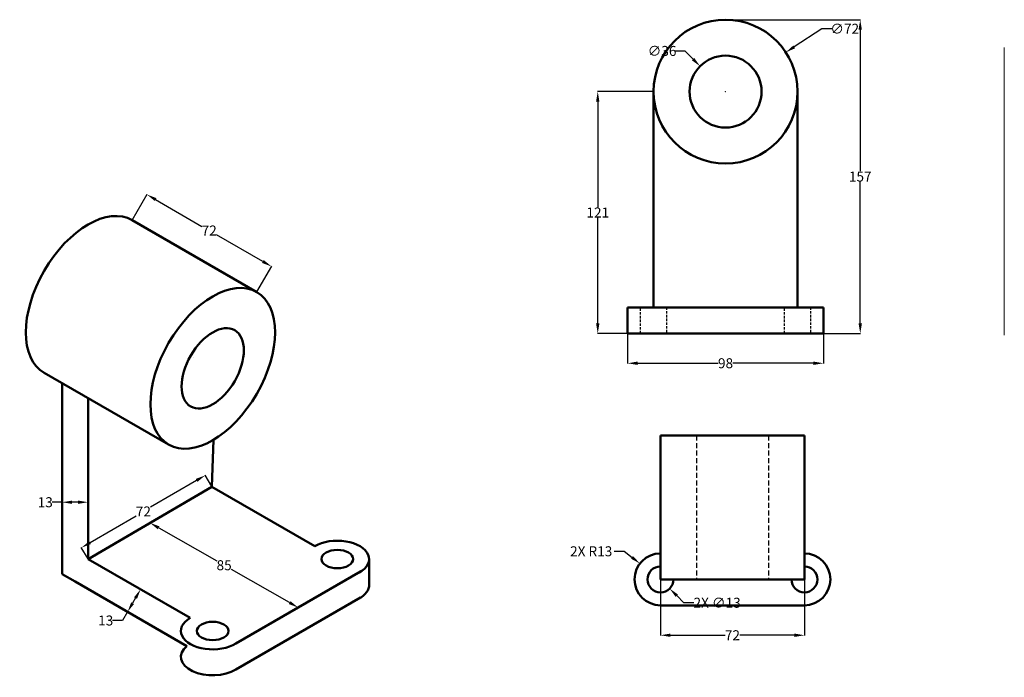
# Model space of a CAD drawing. Units: inches. Extents: x 18 to 510, y -66 to 263.
import ezdxf

# ---------------------------------------------------------------- set-up
doc = ezdxf.new("R2010")
doc.units = ezdxf.units.IN
doc.header["$MEASUREMENT"] = 0
doc.linetypes.add('HIDDEN', pattern=[0.375, 0.25, -0.125])
for name, color, linetype, lineweight in [('M-CONS', 8, 'Continuous', 13), ('M-DIMS', 2, 'Continuous', 25), ('M-HIDN', 7, 'HIDDEN', 25), ('M-OUTL', 7, 'Continuous', 50)]:
    doc.layers.add(name, color=color, linetype=linetype, lineweight=lineweight)
doc.styles.get("Standard").update_dxf_attribs({"font": 'arial.ttf'})
doc.dimstyles.get("Standard").update_dxf_attribs({"dimtxt": 5, "dimasz": 5, "dimexe": 0.18, "dimexo": 0.0625, "dimgap": 0.09, "dimtad": 0, "dimtih": 1, "dimtoh": 1, "dimdec": 0, "dimzin": 0, "dimdsep": 46, "dimtxsty": 'Standard', "dimcen": 0.09, "dimadec": 0, "dimazin": 0, "dimtfac": 1, "dimtdec": 0, "dimtofl": 0, "dimtmove": 0, "dimatfit": 3, "dimfxl": 1, "dimtolj": 1, "dimtzin": 0, "dimarcsym": 0})

# ---------------------------------------------------------------- blocks, each defined once
blk = doc.blocks.new('*D1')
at = {"layer": 'Defpoints', "color": 0, "transparency": 16777216}
for p in [(73.81, 162.95), (143.56, 139.76), (136.17, 126.95)]:
    blk.add_point(p, dxfattribs=at)
at = {"layer": 'M-DIMS', "color": 0, "lineweight": -2, "transparency": 16777216}
for p, q in [((73.84, 163.01), (81.3, 175.91)), ((85.54, 173.26), (108.76, 159.85)), ((139.23, 142.26), (116.01, 155.67)), ((136.2, 127.01), (143.65, 139.91))]:
    blk.add_line(p, q, dxfattribs=at)
at = {"layer": 'M-DIMS', "color": 0, "transparency": 16777216}
for points in [[(85.95, 173.98), (85.12, 172.54), (81.21, 175.76)], [(139.65, 142.98), (138.81, 141.54), (143.56, 139.76)]]:
    blk.add_solid(points, dxfattribs=at)
at = {"layer": 'M-DIMS', "color": 0, "transparency": 16777216, "insert": (112.38, 157.76), "char_height": 5, "attachment_point": 5}
blk.add_mtext('\\A1;72', dxfattribs=at)
blk = doc.blocks.new('*D2')
at = {"layer": 'Defpoints', "color": 0, "transparency": 16777216}
for p in [(38.77, 21.77), (38.77, 21.77), (51.77, 21.77)]:
    blk.add_point(p, dxfattribs=at)
at = {"layer": 'M-DIMS', "color": 0, "lineweight": -2, "transparency": 16777216}
for p, q in [((38.77, 21.77), (33.77, 21.77)), ((38.77, 21.83), (38.77, 21.95)), ((46.77, 21.77), (43.77, 21.77)), ((51.77, 21.83), (51.77, 21.95))]:
    blk.add_line(p, q, dxfattribs=at)
at = {"layer": 'M-DIMS', "color": 0, "transparency": 16777216}
for points in [[(43.77, 22.6), (43.77, 20.94), (38.77, 21.77)], [(46.77, 22.6), (46.77, 20.94), (51.77, 21.77)]]:
    blk.add_solid(points, dxfattribs=at)
at = {"layer": 'M-DIMS', "color": 0, "transparency": 16777216, "insert": (30.33, 21.77), "char_height": 5, "attachment_point": 5}
blk.add_mtext('\\A1;13', dxfattribs=at)
blk = doc.blocks.new('*D3')
at = {"layer": 'Defpoints', "color": 0, "transparency": 16777216}
for p in [(110.41, 35.24), (113.73, 29.55), (51.77, -6.67)]:
    blk.add_point(p, dxfattribs=at)
at = {"layer": 'M-DIMS', "color": 0, "lineweight": -2, "transparency": 16777216}
for p, q in [((113.7, 29.6), (110.32, 35.39)), ((106.09, 32.71), (83.05, 19.25)), ((52.76, 1.54), (75.8, 15.01)), ((51.74, -6.62), (48.35, -0.83))]:
    blk.add_line(p, q, dxfattribs=at)
at = {"layer": 'M-DIMS', "color": 0, "transparency": 16777216}
for points in [[(105.67, 33.43), (106.51, 32), (110.41, 35.24)], [(52.34, 2.26), (53.18, 0.82), (48.44, -0.99)]]:
    blk.add_solid(points, dxfattribs=at)
at = {"layer": 'M-DIMS', "color": 0, "transparency": 16777216, "insert": (79.42, 17.13), "char_height": 5, "attachment_point": 5}
blk.add_mtext('\\A1;72', dxfattribs=at)
blk = doc.blocks.new('*D4')
at = {"layer": 'Defpoints', "color": 0, "transparency": 16777216}
for p in [(82.75, 11.44), (156.93, -30.95), (156.93, -30.95)]:
    blk.add_point(p, dxfattribs=at)
at = {"layer": 'M-DIMS', "color": 0, "lineweight": -2, "transparency": 16777216}
for p, q in [((82.78, 11.49), (82.84, 11.59)), ((87.09, 8.96), (116.15, -7.64)), ((152.59, -28.47), (123.53, -11.87)), ((156.96, -30.89), (157.02, -30.79))]:
    blk.add_line(p, q, dxfattribs=at)
at = {"layer": 'M-DIMS', "color": 0, "transparency": 16777216}
for points in [[(87.5, 9.68), (86.68, 8.23), (82.75, 11.44)], [(153, -27.75), (152.18, -29.19), (156.93, -30.95)]]:
    blk.add_solid(points, dxfattribs=at)
at = {"layer": 'M-DIMS', "color": 0, "transparency": 16777216, "insert": (119.84, -9.76), "char_height": 5, "attachment_point": 5}
blk.add_mtext('\\A1;85', dxfattribs=at)
blk = doc.blocks.new('*D5')
at = {"layer": 'Defpoints', "color": 0, "transparency": 16777216}
for p in [(77.31, -21.42), (70.81, -32.68), (71.53, -33.09)]:
    blk.add_point(p, dxfattribs=at)
at = {"layer": 'M-DIMS', "color": 0, "lineweight": -2, "transparency": 16777216}
for p, q in [((77.37, -21.45), (78.18, -21.92)), ((75.53, -26.16), (74.03, -28.76)), ((71.53, -33.09), (69.03, -37.42)), ((70.87, -32.71), (71.68, -33.18)), ((69.03, -37.42), (64.03, -37.42))]:
    blk.add_line(p, q, dxfattribs=at)
at = {"layer": 'M-DIMS', "color": 0, "transparency": 16777216}
for points in [[(74.81, -25.75), (76.25, -26.58), (78.03, -21.83)], [(73.31, -28.35), (74.75, -29.18), (71.53, -33.09)]]:
    blk.add_solid(points, dxfattribs=at)
at = {"layer": 'M-DIMS', "color": 0, "transparency": 16777216, "insert": (60.59, -37.42), "char_height": 5, "attachment_point": 5}
blk.add_mtext('\\A1;13', dxfattribs=at)
blk = doc.blocks.new('MOUNTING-LUG-PLAN')
for radius, end in [(13, 270), (6.5, 0)]:
    blk.add_arc((13, 13), radius, 90, end)
blk = doc.blocks.new('MOUNTING-HOLE-D13-ELEV')
at = {"ltscale": 5}
for p, q in [((0, 0), (0, 13)), ((13, 13), (13, 0))]:
    blk.add_line(p, q, dxfattribs=at)
blk = doc.blocks.new('MOUNTING-HOLE-D13-ISO')
blk.add_ellipse((7.96, 4.6), major_axis=(-7.96, 0), ratio=0.57735)
blk = doc.blocks.new('*D9')
at = {"layer": 'Defpoints', "color": 0, "transparency": 16777216}
for p in [(321.74, 106.27), (419.74, 106.27), (321.74, 91.32)]:
    blk.add_point(p, dxfattribs=at)
at = {"layer": 'M-DIMS', "color": 0, "lineweight": -2, "transparency": 16777216}
for p, q in [((321.74, 106.21), (321.74, 91.14)), ((419.74, 106.21), (419.74, 91.14)), ((326.74, 91.32), (367.06, 91.32)), ((414.74, 91.32), (374.41, 91.32))]:
    blk.add_line(p, q, dxfattribs=at)
at = {"layer": 'M-DIMS', "color": 0, "transparency": 16777216}
for points in [[(326.74, 92.16), (326.74, 90.49), (321.74, 91.32)], [(414.74, 92.16), (414.74, 90.49), (419.74, 91.32)]]:
    blk.add_solid(points, dxfattribs=at)
at = {"layer": 'M-DIMS', "color": 0, "transparency": 16777216, "insert": (370.74, 91.32), "char_height": 5, "attachment_point": 5}
blk.add_mtext('\\A1;98', dxfattribs=at)
blk = doc.blocks.new('*D10')
at = {"layer": 'Defpoints', "color": 0, "transparency": 16777216}
for p in [(370.74, 263.27), (438.14, 263.27), (419.74, 106.27)]:
    blk.add_point(p, dxfattribs=at)
at = {"layer": 'M-DIMS', "color": 0, "lineweight": -2, "transparency": 16777216}
for p, q in [((370.8, 263.27), (438.32, 263.27)), ((438.14, 258.27), (438.14, 187.42)), ((438.14, 111.27), (438.14, 182.13)), ((419.8, 106.27), (438.32, 106.27))]:
    blk.add_line(p, q, dxfattribs=at)
at = {"layer": 'M-DIMS', "color": 0, "transparency": 16777216}
for points in [[(437.3, 258.27), (438.97, 258.27), (438.14, 263.27)], [(437.3, 111.27), (438.97, 111.27), (438.14, 106.27)]]:
    blk.add_solid(points, dxfattribs=at)
at = {"layer": 'M-DIMS', "color": 0, "transparency": 16777216, "insert": (438.14, 184.77), "char_height": 5, "attachment_point": 5}
blk.add_mtext('\\A1;157', dxfattribs=at)
blk = doc.blocks.new('*D11')
at = {"layer": 'Defpoints', "color": 0, "transparency": 16777216}
for p in [(306.79, 227.27), (334.74, 227.27), (321.74, 106.27)]:
    blk.add_point(p, dxfattribs=at)
at = {"layer": 'M-DIMS', "color": 0, "lineweight": -2, "transparency": 16777216}
for p, q in [((334.67, 227.27), (306.61, 227.27)), ((306.79, 222.27), (306.79, 169.37)), ((306.79, 111.27), (306.79, 164.17)), ((321.67, 106.27), (306.61, 106.27))]:
    blk.add_line(p, q, dxfattribs=at)
at = {"layer": 'M-DIMS', "color": 0, "transparency": 16777216}
for points in [[(305.95, 222.27), (307.62, 222.27), (306.79, 227.27)], [(305.95, 111.27), (307.62, 111.27), (306.79, 106.27)]]:
    blk.add_solid(points, dxfattribs=at)
at = {"layer": 'M-DIMS', "color": 0, "transparency": 16777216, "insert": (306.79, 166.77), "char_height": 5, "attachment_point": 5}
blk.add_mtext('\\A1;121', dxfattribs=at)
blk = doc.blocks.new('*D12')
at = {"layer": 'Defpoints', "color": 0, "transparency": 16777216}
for p in [(338.19, -16.85), (410.19, -16.85), (410.19, -44.8)]:
    blk.add_point(p, dxfattribs=at)
at = {"layer": 'M-DIMS', "color": 0, "lineweight": -2, "transparency": 16777216}
for p, q in [((338.19, -16.92), (338.19, -44.98)), ((410.19, -16.92), (410.19, -44.98)), ((343.19, -44.8), (370.56, -44.8)), ((405.19, -44.8), (377.81, -44.8))]:
    blk.add_line(p, q, dxfattribs=at)
at = {"layer": 'M-DIMS', "color": 0, "transparency": 16777216}
for points in [[(343.19, -43.97), (343.19, -45.64), (338.19, -44.8)], [(405.19, -43.97), (405.19, -45.64), (410.19, -44.8)]]:
    blk.add_solid(points, dxfattribs=at)
at = {"layer": 'M-DIMS', "color": 0, "transparency": 16777216, "insert": (374.19, -44.8), "char_height": 5, "attachment_point": 5}
blk.add_mtext('\\A1;72', dxfattribs=at)
blk = doc.blocks.new('*D13')
at = {"layer": 'Defpoints', "color": 0, "transparency": 16777216}
for p in [(400.9, 246.93), (340.58, 207.61)]:
    blk.add_point(p, dxfattribs=at)
at = {"layer": 'M-DIMS', "color": 0, "lineweight": -2, "transparency": 16777216}
for p, q in [((418.99, 258.73), (405.08, 249.66)), ((423.99, 258.73), (418.99, 258.73)), ((370.65, 227.27), (370.83, 227.27)), ((370.74, 227.18), (370.74, 227.36))]:
    blk.add_line(p, q, dxfattribs=at)
at = {"layer": 'M-DIMS', "color": 0, "transparency": 16777216}
blk.add_solid([(404.63, 250.36), (405.54, 248.96), (400.9, 246.93)], dxfattribs=at)
at = {"layer": 'M-DIMS', "color": 0, "transparency": 16777216, "insert": (430.36, 258.73), "char_height": 5, "attachment_point": 5}
blk.add_mtext('\\A1;∅72', dxfattribs=at)
blk = doc.blocks.new('*D14')
at = {"layer": 'Defpoints', "color": 0, "transparency": 16777216}
for p in [(358, 240), (383.47, 214.55)]:
    blk.add_point(p, dxfattribs=at)
at = {"layer": 'M-DIMS', "color": 0, "lineweight": -2, "transparency": 16777216}
for p, q in [((345.36, 247.63), (350.36, 247.63)), ((350.36, 247.63), (354.47, 243.53)), ((370.65, 227.27), (370.83, 227.27)), ((370.74, 227.18), (370.74, 227.36))]:
    blk.add_line(p, q, dxfattribs=at)
at = {"layer": 'M-DIMS', "color": 0, "transparency": 16777216}
blk.add_solid([(355.06, 244.12), (353.88, 242.94), (358, 240)], dxfattribs=at)
at = {"layer": 'M-DIMS', "color": 0, "transparency": 16777216, "insert": (338.98, 247.63), "char_height": 5, "attachment_point": 5}
blk.add_mtext('\\A1;∅36', dxfattribs=at)
blk = doc.blocks.new('*D15')
at = {"layer": 'Defpoints', "color": 0, "transparency": 16777216}
for p in [(327.9, -8.9), (338.19, -16.85)]:
    blk.add_point(p, dxfattribs=at)
at = {"layer": 'M-DIMS', "color": 0, "lineweight": -2, "transparency": 16777216}
for p, q in [((314.99, -2.79), (319.99, -2.79)), ((319.99, -2.79), (323.95, -5.84)), ((338.1, -16.85), (338.28, -16.85)), ((338.19, -16.94), (338.19, -16.76))]:
    blk.add_line(p, q, dxfattribs=at)
at = {"layer": 'M-DIMS', "color": 0, "transparency": 16777216}
blk.add_solid([(324.46, -5.19), (323.44, -6.5), (327.9, -8.9)], dxfattribs=at)
at = {"layer": 'M-DIMS', "color": 0, "transparency": 16777216, "insert": (303.51, -2.79), "char_height": 5, "attachment_point": 5}
blk.add_mtext('\\A1;2X R13', dxfattribs=at)
blk = doc.blocks.new('*D16')
at = {"layer": 'Defpoints', "color": 0, "transparency": 16777216}
for p in [(333.59, -12.26), (342.78, -21.45)]:
    blk.add_point(p, dxfattribs=at)
at = {"layer": 'M-DIMS', "color": 0, "lineweight": -2, "transparency": 16777216}
for p, q in [((338.1, -16.85), (338.28, -16.85)), ((338.19, -16.94), (338.19, -16.76)), ((349.85, -28.53), (346.32, -24.99)), ((354.85, -28.53), (349.85, -28.53))]:
    blk.add_line(p, q, dxfattribs=at)
at = {"layer": 'M-DIMS', "color": 0, "transparency": 16777216}
blk.add_solid([(346.91, -24.4), (345.73, -25.58), (342.78, -21.45)], dxfattribs=at)
at = {"layer": 'M-DIMS', "color": 0, "transparency": 16777216, "insert": (366.52, -28.53), "char_height": 5, "attachment_point": 5}
blk.add_mtext('\\A1;2X ∅13', dxfattribs=at)

msp = doc.modelspace()

# ---------------------------------------------------------------- linework, layer by layer
at = {"layer": 'M-CONS'}
for p, q in [((510.22, 213.33), (510.22, 249.33)), ((510.22, 105.33), (510.22, 213.33)), ((104.35, 94.41), (104.35, 94.41)), ((104.35, 94.41), (104.35, 94.41))]:
    msp.add_line(p, q, dxfattribs=at)
at = {"layer": 'M-HIDN', "ltscale": 10}
for p, q in [((356.19, 55.15), (356.19, -16.85)), ((392.19, 55.15), (392.19, -16.85))]:
    msp.add_line(p, q, dxfattribs=at)
at = {"layer": 'M-OUTL'}
for p, q in [((334.74, 227.27), (334.74, 119.27)), ((406.74, 119.27), (406.74, 227.27)), ((136.17, 126.95), (73.81, 162.95)), ((73.81, 162.95), (136.17, 126.95)), ((321.74, 106.27), (321.74, 119.27)), ((321.74, 119.27), (334.74, 119.27)), ((334.74, 119.27), (406.74, 119.27)), ((334.74, 119.27), (341.24, 119.27)), ((406.74, 119.27), (400.24, 119.27)), ((406.74, 119.27), (419.74, 119.27)), ((406.74, 119.27), (413.24, 119.27)), ((419.74, 119.27), (419.74, 106.27)), ((419.74, 106.27), (321.74, 106.27)), ((341.24, 106.27), (328.24, 106.27)), ((92.08, 50.58), (29.72, 86.58)), ((38.77, -14.18), (38.77, 81.36)), ((51.77, -6.67), (51.77, 73.86)), ((338.19, 55.15), (410.19, 55.15)), ((338.19, -16.85), (338.19, 55.15)), ((410.19, 55.15), (410.19, -16.85)), ((113.73, 29.55), (114.5, 52.99)), ((51.77, -6.67), (113.73, 29.55)), ((113.73, 29.55), (165.22, -0.17)), ((51.77, -6.67), (102.86, -36.17)), ((102.86, -36.17), (51.77, -6.67)), ((102.86, -36.17), (51.77, -6.67)), ((192.39, -19.89), (192.4, -6.68)), ((45.27, -17.93), (38.77, -14.18)), ((125.75, -48.95), (188.11, -12.95)), ((101.26, -50.26), (45.27, -17.93)), ((410.19, -16.85), (338.19, -16.85)), ((125.75, -61.95), (188.11, -25.95)), ((410.19, -29.85), (338.19, -29.85))]:
    msp.add_line(p, q, dxfattribs=at)
for radius in [36, 18]:
    msp.add_circle((370.74, 227.27), radius, dxfattribs=at)
for centre, major_axis, start_param, end_param in [((51.77, 124.77), (-22.05, -38.18), 3.141593, 6.283185), ((176.47, -6.67), (-15.92, 0), 2.322276, 5.497787), ((176.47, -19.67), (-15.92, 0), 3.926991, 3.927566), ((176.47, -19.67), (-15.92, 0), 2.322276, 3.164974), ((114.12, -42.67), (-15.92, 0), 5.497787, 8.673298), ((114.12, -55.67), (-15.92, 0), 5.653111, 8.673298)]:
    msp.add_ellipse(centre, major_axis=major_axis, ratio=0.57735, start_param=start_param, end_param=end_param, dxfattribs=at)
for major_axis in [(-22.05, -38.18), (-11.02, -19.09)]:
    msp.add_ellipse((114.12, 88.77), major_axis=major_axis, ratio=0.57735, dxfattribs=at)

# ---------------------------------------------------------------- block references
at = {"layer": 'M-HIDN'}
for p in [(328.24, 106.27), (400.24, 106.27)]:
    msp.add_blockref('MOUNTING-HOLE-D13-ELEV', p, dxfattribs=at)
at = {"layer": 'M-OUTL'}
for name, p in [('MOUNTING-HOLE-D13-ISO', (168.51, -11.27)), ('MOUNTING-LUG-PLAN', (325.19, -29.85)), ('MOUNTING-HOLE-D13-ISO', (106.16, -47.27))]:
    msp.add_blockref(name, p, dxfattribs=at)
at = {"layer": 'M-OUTL', "extrusion": (0, 0, -1), "zscale": -1}
msp.add_blockref('MOUNTING-LUG-PLAN', (-423.19, -29.85), dxfattribs=at)

# ---------------------------------------------------------------- dimensions: what is measured, and where the dimension line sits
at = {"layer": 'M-DIMS'}
for p1, p2, picture, middle in [((340.58, 207.61), (400.9, 246.93), '*D13', (430.36, 258.73)), ((383.47, 214.55), (358, 240), '*D14', (338.98, 247.63))]:
    dim = msp.add_diameter_dim_2p(p1=p1, p2=p2, dimstyle='Standard', override={"dimdec": 0, "dimlfac": 1, "dimrnd": 0, "dimzin": 0, "dimdsep": 46, "dimlunit": 2}, dxfattribs=at)
    dim.commit()
    dim.dimension.update_dxf_attribs({"geometry": picture, "text_midpoint": middle, "dimtype": 163})
for base, p1, p2, angle, picture, middle in [((438.14, 263.27), (419.74, 106.27), (370.74, 263.27), 90, '*D10', (438.14, 184.77)), ((306.79, 227.27), (321.74, 106.27), (334.74, 227.27), 90, '*D11', (306.79, 166.77)), ((321.74, 91.32), (419.74, 106.27), (321.74, 106.27), 180, '*D9', (370.74, 91.32))]:
    dim = msp.add_linear_dim(base=base, p1=p1, p2=p2, angle=angle, dimstyle='Standard', override={"dimdec": 0, "dimlfac": 1, "dimrnd": 0, "dimzin": 0, "dimdsep": 46, "dimlunit": 2}, dxfattribs=at)
    dim.commit()
    dim.dimension.update_dxf_attribs({"geometry": picture, "text_midpoint": middle})
for p1, p2, distance, picture, middle in [((73.81, 162.95), (136.17, 126.95), 14.79, '*D1', (112.38, 157.76)), ((51.77, -6.67), (113.73, 29.55), 6.59, '*D3', (79.42, 17.13)), ((51.77, 21.77), (38.77, 21.77), 0, '*D2', (30.33, 21.77)), ((82.75, 11.44), (156.93, -30.95), 0, '*D4', (119.84, -9.76)), ((77.31, -21.42), (70.81, -32.68), 0.82, '*D5', (60.59, -37.42))]:
    dim = msp.add_aligned_dim(p1=p1, p2=p2, distance=distance, dimstyle='Standard', override={"dimclrd": 0, "dimclre": 0, "dimclrt": 0}, dxfattribs=at)
    dim.commit()
    dim.dimension.update_dxf_attribs({"geometry": picture, "text_midpoint": middle})
dim = msp.add_radius_dim(center=(338.19, -16.85), mpoint=(327.9, -8.9), text='2X <>', dimstyle='Standard', override={"dimdec": 0, "dimlfac": 1, "dimrnd": 0, "dimzin": 0, "dimdsep": 46, "dimlunit": 2}, dxfattribs=at)
dim.commit()
dim.dimension.update_dxf_attribs({"geometry": '*D15', "text_midpoint": (303.51, -2.79)})
dim = msp.add_diameter_dim_2p(p1=(333.59, -12.26), p2=(342.78, -21.45), text='2X <>', dimstyle='Standard', override={"dimdec": 0, "dimlfac": 1, "dimrnd": 0, "dimzin": 0, "dimdsep": 46, "dimlunit": 2}, dxfattribs=at)
dim.commit()
dim.dimension.update_dxf_attribs({"geometry": '*D16', "text_midpoint": (366.52, -28.53), "dimtype": 163})
dim = msp.add_linear_dim(base=(410.19, -44.8), p1=(338.19, -16.85), p2=(410.19, -16.85), dimstyle='Standard', override={"dimdec": 0, "dimlfac": 1, "dimrnd": 0, "dimzin": 0, "dimdsep": 46, "dimlunit": 2}, dxfattribs=at)
dim.commit()
dim.dimension.update_dxf_attribs({"geometry": '*D12', "text_midpoint": (374.19, -44.8)})

doc.saveas('drawing.dxf')
